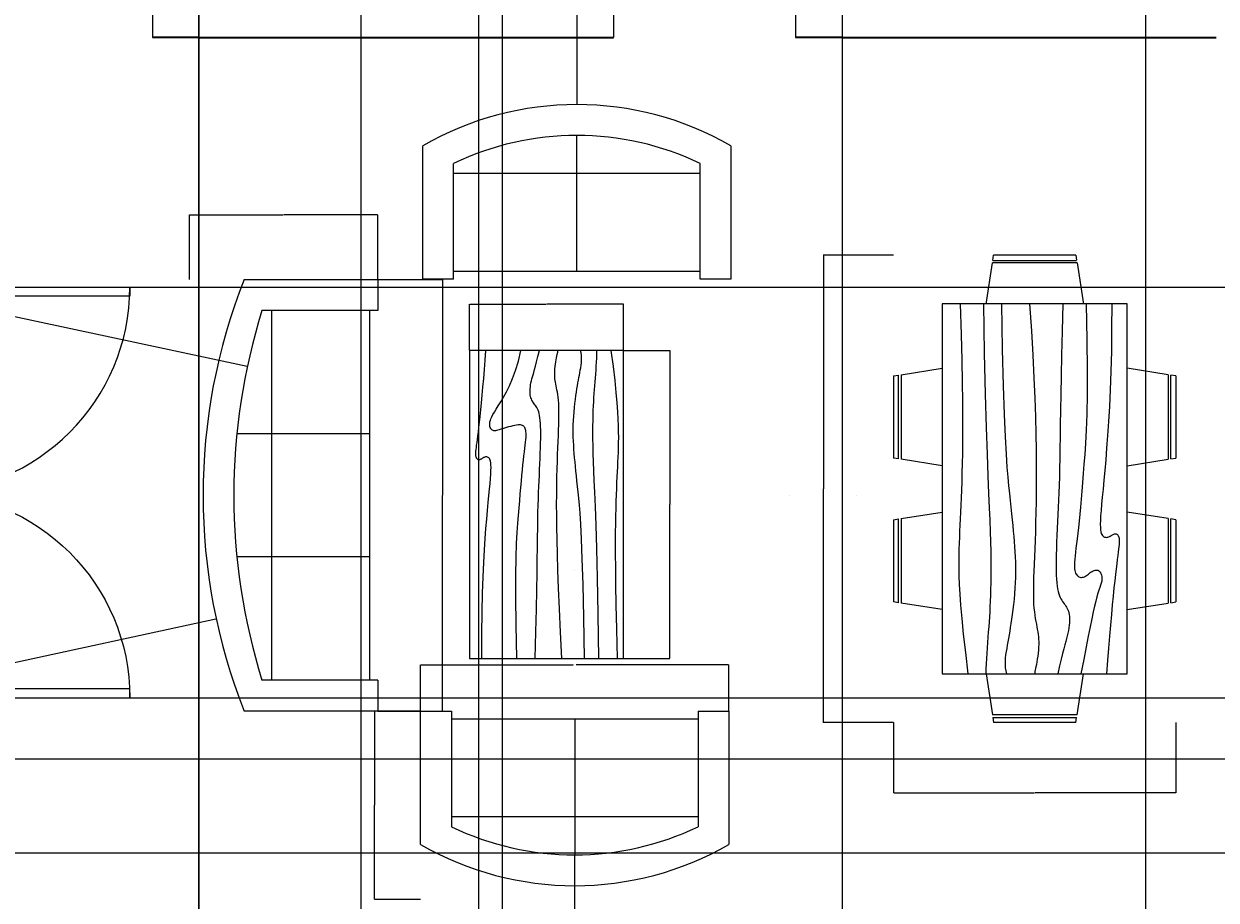
# Model space of a CAD drawing. Units: millimetres. Extents: x -8052 to 19968, y -37825 to -17505.
# Tile 4 of 10: x 84 to 5980, y -29741 to -25407. Entities that reach past the tile are written whole.
import ezdxf

# ---------------------------------------------------------------- set-up
doc = ezdxf.new("R2010")
doc.units = ezdxf.units.MM
doc.header["$MEASUREMENT"] = 0
for name, color, linetype, lineweight in [('A-ANNO-DIMS', 2, 'Continuous', 18), ('A-DOOR', 3, 'Continuous', 25), ('A-FURN', 8, 'Continuous', 18), ('A-WALL', 7, 'Continuous', 35)]:
    doc.layers.add(name, color=color, linetype=linetype, lineweight=lineweight)
doc.styles.get("Standard").update_dxf_attribs({"font": 'arial.ttf'})
doc.dimstyles.get("Standard").update_dxf_attribs({"dimtxt": 1.054, "dimasz": 1.055, "dimexe": 0.18, "dimexo": 0.0625, "dimgap": 0.09, "dimtad": 0, "dimtih": 1, "dimtoh": 1, "dimdec": 4, "dimzin": 0, "dimdsep": 46, "dimtxsty": 'Standard', "dimcen": 0.09, "dimadec": 0, "dimazin": 0, "dimtfac": 1, "dimtdec": 4, "dimtofl": 0, "dimtmove": 0, "dimatfit": 3, "dimfxl": 1, "dimtolj": 1, "dimtzin": 0, "dimarcsym": 0})

# ---------------------------------------------------------------- blocks, each defined once
blk = doc.blocks.new('Dining Set - 36 x 72 in.')
for p, q in [((-22.2343, 26.00059), (-23.4847, 17.99762)), ((-22.2304, 26), (-5.7608, 26)), ((-22, 27.5), (-22.1562, 26.50042)), ((-5.8416, 26.5), (-22.1534, 26.5)), ((-22, 27.5), (-6, 27.5)), ((-5.8437, 26.49966), (-6, 27.5)), ((-4.5152, 17.99762), (-5.7655, 25.99926)), ((5.7657, 26.00059), (4.5153, 17.99762)), ((5.7696, 26), (22.2392, 26)), ((6, 27.5), (5.8438, 26.50042)), ((22.1584, 26.5), (5.8466, 26.5)), ((6, 27.5), (22, 27.5)), ((22.1563, 26.49966), (22, 27.5)), ((23.4848, 17.99762), (22.2345, 25.99926)), ((36, 18), (-36, 18)), ((-36, 18), (-36, -18)), ((36, -18), (36, 18)), ((-44.0006, 8.23428), (-35.9976, 9.48474)), ((44.0006, 8.23428), (35.9976, 9.48474)), ((-45.5, 8), (-44.5004, 8.15617)), ((-45.5, 8), (-45.5, -8)), ((-44.5, -8.15843), (-44.5, 8.15338)), ((-44, 8.23041), (-44, -8.23915)), ((44, 8.23041), (44, -8.23915)), ((44.5, -8.15843), (44.5, 8.15338)), ((45.5, 8), (44.5005, 8.15617)), ((45.5, 8), (45.5, -8)), ((-44.4997, -8.15631), (-45.5, -8)), ((-35.9976, -9.48476), (-43.9993, -8.2345)), ((35.9976, -9.48476), (43.9993, -8.2345)), ((44.4997, -8.15631), (45.5, -8)), ((-36, -18), (36, -18)), ((-22.2343, -26.0006), (-23.4847, -17.99762)), ((-4.5152, -17.99762), (-5.7655, -25.99928)), ((5.7657, -26.0006), (4.5153, -17.99762)), ((23.4848, -17.99762), (22.2345, -25.99928)), ((-22.2304, -26), (-5.7608, -26)), ((-22, -27.5), (-22.1562, -26.50044)), ((-5.8416, -26.5), (-22.1534, -26.5)), ((-22, -27.5), (-6, -27.5)), ((-5.8437, -26.49967), (-6, -27.5)), ((5.7696, -26), (22.2392, -26)), ((6, -27.5), (5.8438, -26.50044)), ((22.1584, -26.5), (5.8466, -26.5)), ((6, -27.5), (22, -27.5)), ((22.1563, -26.49967), (22, -27.5))]:
    blk.add_line(p, q)
for points in [[(-36, 15), (-31.1772, 14.97754), (-26.8079, 14.91406), (-22.8538, 14.81543), (-19.276, 14.6875), (-16.0362, 14.53613), (-13.0957, 14.36718), (-10.4159, 14.18652), (-7.9583, 14), (-5.6904, 13.81315), (-3.6035, 13.63021), (-1.6954, 13.45508), (0.0365, 13.29166), (1.5945, 13.14388), (2.9811, 13.01562), (4.1988, 12.9108), (5.25, 12.83333), (6.1393, 12.78613), (6.8802, 12.76823), (7.4883, 12.77767), (7.9792, 12.8125), (8.3685, 12.87077), (8.6719, 12.95052), (8.9049, 13.0498), (9.0833, 13.16666), (9.2205, 13.29899), (9.3216, 13.44401), (9.3895, 13.59879), (9.4271, 13.76041), (9.4373, 13.92594), (9.4232, 14.09245), (9.3875, 14.257), (9.3333, 14.41666), (9.2638, 14.56917), (9.1836, 14.71484), (9.0975, 14.85465), (9.0104, 14.98958), (8.9272, 15.1206), (8.8529, 15.2487), (8.7922, 15.37483), (8.75, 15.5), (8.7305, 15.62467), (8.7344, 15.74739), (8.7617, 15.86621), (8.8125, 15.97916), (8.8867, 16.08431), (8.9844, 16.17968), (9.1055, 16.26334), (9.25, 16.33333), (9.4189, 16.38802), (9.6172, 16.42708), (9.8506, 16.45052), (10.125, 16.45833), (10.4463, 16.45052), (10.8203, 16.42708), (11.2529, 16.38802), (11.75, 16.33333), (12.3184, 16.26318), (12.9694, 16.17838), (13.7151, 16.07991), (14.5677, 15.96875), (15.5395, 15.84586), (16.6426, 15.71224), (17.8893, 15.56884), (19.2917, 15.41666), (20.859, 15.25667), (22.5879, 15.08984), (24.4721, 14.91715), (26.5052, 14.73958), (28.6809, 14.5581), (30.9929, 14.3737), (33.4347, 14.18733), (36, 14)], [(-36, 10), (-28.9766, 10.14274), (-23.1725, 10.20442), (-18.4241, 10.19775), (-14.5677, 10.13541), (-11.4399, 10.03011), (-8.877, 9.89453), (-6.7154, 9.74137), (-4.7917, 9.58333), (-2.9698, 9.43082), (-1.2246, 9.28515), (0.4415, 9.14534), (2.026, 9.01041), (3.5266, 8.87939), (4.9408, 8.7513), (6.266, 8.62516), (7.5, 8.5), (8.6411, 8.37549), (9.6914, 8.2539), (10.6538, 8.13818), (11.5312, 8.03125), (12.3267, 7.93603), (13.043, 7.85547), (13.6831, 7.79248), (14.25, 7.75), (14.7471, 7.7303), (15.1797, 7.73307), (15.5537, 7.75732), (15.875, 7.80208), (16.1494, 7.86637), (16.3828, 7.94922), (16.5811, 8.04964), (16.75, 8.16666), (16.8944, 8.29915), (17.0143, 8.44531), (17.1089, 8.60319), (17.1771, 8.77083), (17.218, 8.94629), (17.2305, 9.1276), (17.2137, 9.31282), (17.1667, 9.5), (17.0895, 9.6875), (16.987, 9.875), (16.8649, 10.0625), (16.7292, 10.25), (16.5856, 10.4375), (16.4401, 10.625), (16.2985, 10.8125), (16.1667, 11), (16.05, 11.18733), (15.9518, 11.3737), (15.8752, 11.5581), (15.8229, 11.73958), (15.798, 11.91715), (15.8034, 12.08984), (15.842, 12.25667), (15.9167, 12.41666), (16.0295, 12.56836), (16.1784, 12.70833), (16.3605, 12.83268), (16.5729, 12.9375), (16.8127, 13.01888), (17.0768, 13.07291), (17.3625, 13.0957), (17.6667, 13.08333), (17.9894, 13.03312), (18.3418, 12.94726), (18.7382, 12.82918), (19.1927, 12.68229), (19.7195, 12.51001), (20.3327, 12.31575), (21.0465, 12.10294), (21.875, 11.875), (22.8357, 11.63354), (23.959, 11.37304), (25.2786, 11.08618), (26.8282, 10.76562), (28.6414, 10.40405), (30.752, 9.99414), (33.1936, 9.52856), (36, 9)], [(-36, 5.5), (-30.7157, 5.3348), (-26.069, 5.20963), (-21.9946, 5.11767), (-18.4271, 5.05208), (-15.3009, 5.00602), (-12.5508, 4.97265), (-10.1112, 4.94515), (-7.9167, 4.91666), (-5.909, 4.88167), (-4.0586, 4.83984), (-2.3429, 4.79215), (-0.7396, 4.73958), (0.7739, 4.6831), (2.22, 4.6237), (3.6213, 4.56233), (5, 4.5), (6.373, 4.43782), (7.7344, 4.3776), (9.0723, 4.32129), (10.375, 4.27083), (11.6309, 4.22819), (12.8281, 4.19531), (13.9551, 4.17415), (15, 4.16666), (15.954, 4.17448), (16.819, 4.19791), (17.6001, 4.23698), (18.3021, 4.29166), (18.9299, 4.36198), (19.4883, 4.44791), (19.9823, 4.54948), (20.4167, 4.66666), (20.7969, 4.79899), (21.1302, 4.94401), (21.4245, 5.09879), (21.6875, 5.26041), (21.9271, 5.42594), (22.1511, 5.59245), (22.3672, 5.757), (22.5834, 5.91666), (22.8065, 6.06868), (23.0404, 6.21093), (23.2879, 6.34147), (23.5521, 6.45833), (23.8358, 6.55957), (24.142, 6.64323), (24.4735, 6.70735), (24.8334, 6.75), (25.2235, 6.76969), (25.642, 6.76692), (26.0858, 6.74267), (26.5521, 6.69791), (27.0379, 6.63362), (27.5404, 6.55078), (28.0565, 6.45036), (28.5834, 6.33333), (29.1242, 6.19987), (29.7071, 6.04687), (30.3661, 5.87044), (31.1354, 5.66666), (32.0493, 5.43164), (33.142, 5.16146), (34.4475, 4.85221), (36, 4.5)], [(-36, -1), (-30.7915, -0.6591), (-26.0195, -0.38216), (-21.6519, -0.16284), (-17.6563, 0.00521), (-14.0005, 0.12833), (-10.6523, 0.21289), (-7.5796, 0.26522), (-4.75, 0.29166), (-2.134, 0.29793), (0.2878, 0.28711), (2.5317, 0.26163), (4.6146, 0.22396), (6.5529, 0.17651), (8.3633, 0.12174), (10.0623, 0.06209), (11.6667, 0), (13.1899, -0.06201), (14.6341, -0.1211), (15.9982, -0.17432), (17.2813, -0.21875), (18.4823, -0.25147), (19.6003, -0.26953), (20.6343, -0.27002), (21.5834, -0.25), (22.4481, -0.20768), (23.2357, -0.14584), (23.9549, -0.06836), (24.6146, 0.02083), (25.2235, 0.11784), (25.7904, 0.21875), (26.3241, 0.31966), (26.8334, 0.41666), (27.3265, 0.50618), (27.8099, 0.58593), (28.2894, 0.65397), (28.7709, 0.70833), (29.2601, 0.74707), (29.763, 0.76823), (30.2855, 0.76985), (30.8334, 0.75), (31.4088, 0.70784), (31.9994, 0.64713), (32.589, 0.57275), (33.1615, 0.48958), (33.7008, 0.4025), (34.1908, 0.3164), (34.6153, 0.23616), (34.9584, 0.16666), (35.2099, 0.11165), (35.3848, 0.07031), (35.504, 0.04069), (35.5886, 0.02083), (35.6594, 0.00879), (35.7377, 0.0026), (35.8442, 0.00032), (36, 0)], [(-36, -6.5), (-27.1843, -6.31267), (-20.084, -6.1263), (-14.469, -5.9419), (-10.1094, -5.76042), (-6.7752, -5.58285), (-4.2363, -5.41016), (-2.2629, -5.24333), (-0.625, -5.08334), (0.8708, -4.93099), (2.2715, -4.78646), (3.5872, -4.64974), (4.8281, -4.52084), (6.0046, -4.39974), (7.127, -4.28646), (8.2053, -4.18099), (9.25, -4.08334), (10.2705, -3.99382), (11.2734, -3.91407), (12.2647, -3.84603), (13.25, -3.79167), (14.2354, -3.75293), (15.2266, -3.73177), (16.2295, -3.73015), (17.25, -3.75), (18.2912, -3.79248), (19.3451, -3.85547), (20.4009, -3.93604), (21.4479, -4.03125), (22.4754, -4.13819), (23.4727, -4.25391), (24.4289, -4.37549), (25.3334, -4.5), (26.1785, -4.62492), (26.9694, -4.74935), (27.7145, -4.87281), (28.4219, -4.99479), (29.1, -5.11483), (29.7572, -5.23242), (30.4016, -5.34709), (31.0417, -5.45834), (31.6837, -5.56437), (32.3262, -5.65821), (32.9658, -5.73153), (33.599, -5.77604), (34.2224, -5.78345), (34.8327, -5.74545), (35.4264, -5.65373), (36, -5.5)], [(-36, -10), (-26.4022, -9.81299), (-18.4675, -9.62891), (-11.9839, -9.45069), (-6.7396, -9.28125), (-2.5226, -9.12354), (0.8789, -8.98047), (3.6769, -8.85498), (6.0833, -8.75), (8.2767, -8.66765), (10.3021, -8.60677), (12.1712, -8.56543), (13.8958, -8.54167), (15.4876, -8.53353), (16.9583, -8.53907), (18.3197, -8.55632), (19.5834, -8.58334), (20.7616, -8.61841), (21.8685, -8.66081), (22.9188, -8.71004), (23.9271, -8.76563), (24.9081, -8.82707), (25.8763, -8.89388), (26.8465, -8.96558), (27.8334, -9.04167), (28.8474, -9.12118), (29.8828, -9.20117), (30.93, -9.27824), (31.9792, -9.34896), (33.0205, -9.40991), (34.0443, -9.45768), (35.0407, -9.48885), (36, -9.5)], [(-36, -14.5), (-30.0881, -14.33513), (-25.0332, -14.21224), (-20.7312, -14.12647), (-17.0781, -14.07292), (-13.97, -14.04671), (-11.3027, -14.04297), (-8.9724, -14.05681), (-6.875, -14.08334), (-4.9224, -14.11833), (-3.0905, -14.16016), (-1.3709, -14.20785), (0.2448, -14.26042), (1.7647, -14.3169), (3.1973, -14.3763), (4.5507, -14.43767), (5.8333, -14.5), (7.0554, -14.5621), (8.235, -14.62175), (9.3922, -14.67652), (10.5469, -14.72396), (11.7192, -14.76164), (12.929, -14.78711), (14.1965, -14.79794), (15.5417, -14.79167), (16.9933, -14.76424), (18.6152, -14.70508), (20.4804, -14.60197), (22.6615, -14.44271), (25.2312, -14.21509), (28.2624, -13.9069), (31.8277, -13.50594), (36, -13)]]:
    blk.add_lwpolyline(points)
blk = doc.blocks.new('Table - Rectangular Woodgrain 60 x 30 in.')
for p, q in [((0, 0), (0, -30)), ((60, 0), (0, 0)), ((60, -30), (60, 0)), ((0, -30), (60, -30))]:
    blk.add_line(p, q)
for points in [[(0, -2.4), (4.8155, -2.418), (9.0302, -2.4688), (12.709, -2.5477), (15.9167, -2.65), (18.7181, -2.7711), (21.1781, -2.9063), (23.3616, -3.0508), (25.3333, -3.2), (27.1477, -3.3495), (28.8172, -3.4958), (30.3437, -3.636), (31.7291, -3.7667), (32.9756, -3.8849), (34.0849, -3.9875), (35.059, -4.0714), (35.9, -4.1334), (36.6114, -4.1711), (37.2041, -4.1854), (37.6906, -4.1779), (38.0833, -4.15), (38.3948, -4.1034), (38.6375, -4.0396), (38.8239, -3.9602), (38.9666, -3.8667), (39.0764, -3.7608), (39.1573, -3.6448), (39.2116, -3.521), (39.2416, -3.3917), (39.2498, -3.2593), (39.2385, -3.1261), (39.21, -2.9944), (39.1666, -2.8667), (39.111, -2.7447), (39.0468, -2.6281), (38.978, -2.5163), (38.9083, -2.4083), (38.8418, -2.3035), (38.7823, -2.201), (38.7337, -2.1001), (38.7, -2), (38.6844, -1.9003), (38.6875, -1.8021), (38.7094, -1.707), (38.75, -1.6167), (38.8094, -1.5326), (38.8875, -1.4563), (38.9844, -1.3893), (39.1, -1.3333), (39.2351, -1.2896), (39.3937, -1.2583), (39.5804, -1.2396), (39.8, -1.2333), (40.057, -1.2396), (40.3562, -1.2583), (40.7023, -1.2896), (41.1, -1.3333), (41.5547, -1.3895), (42.0755, -1.4573), (42.6721, -1.5361), (43.3542, -1.625), (44.1316, -1.7233), (45.014, -1.8302), (46.0114, -1.9449), (47.1333, -2.0667), (48.3862, -2.1947), (49.7625, -2.3281), (51.2513, -2.4663), (52.8416, -2.6083), (54.5226, -2.7535), (56.2833, -2.9011), (58.1127, -3.0501), (60, -3.2)], [(0, -9.2), (6.5759, -9.0858), (11.9385, -9.0365), (16.2527, -9.0418), (19.6833, -9.0917), (22.3952, -9.1759), (24.5531, -9.2844), (26.322, -9.4069), (27.8666, -9.5333), (29.3241, -9.6553), (30.7203, -9.7719), (32.0532, -9.8837), (33.3208, -9.9917), (34.5213, -10.0965), (35.6526, -10.199), (36.7128, -10.2999), (37.7, -10.4), (38.6129, -10.4996), (39.4531, -10.5969), (40.223, -10.6895), (40.925, -10.775), (41.5613, -10.8512), (42.1344, -10.9156), (42.6465, -10.966), (43.1, -11), (43.4976, -11.0158), (43.8437, -11.0136), (44.143, -10.9942), (44.4, -10.9583), (44.6195, -10.9069), (44.8062, -10.8406), (44.9648, -10.7603), (45.1, -10.6667), (45.2155, -10.5598), (45.3114, -10.4365), (45.3871, -10.2929), (45.4416, -10.125), (45.4743, -9.929), (45.4844, -9.7011), (45.4709, -9.4371), (45.4333, -9.1333), (45.3716, -8.7883), (45.2896, -8.4104), (45.1919, -8.0107), (45.0833, -7.6), (44.9685, -7.1893), (44.8521, -6.7896), (44.7388, -6.4117), (44.6333, -6.0667), (44.54, -5.7628), (44.4614, -5.4979), (44.4001, -5.2675), (44.3583, -5.0667), (44.3384, -4.8909), (44.3427, -4.7354), (44.3736, -4.5956), (44.4333, -4.4667), (44.5236, -4.3453), (44.6427, -4.2333), (44.7884, -4.1339), (44.9583, -4.05), (45.1501, -3.9849), (45.3614, -3.9417), (45.59, -3.9234), (45.8333, -3.9333), (46.0915, -3.9749), (46.3734, -4.0531), (46.6906, -4.1736), (47.0542, -4.3417), (47.4756, -4.5629), (47.9661, -4.8427), (48.5372, -5.1866), (49.2, -5.6), (49.9676, -6.0844), (50.8594, -6.625), (51.8965, -7.2031), (53.1, -7.8), (54.491, -8.3969), (56.0906, -8.975), (57.9199, -9.5156), (60, -10)], [(0, -12.8), (5.1847, -12.9322), (9.6213, -13.0323), (13.3963, -13.1059), (16.5958, -13.1583), (19.3063, -13.1952), (21.614, -13.2219), (23.6054, -13.2439), (25.3666, -13.2667), (26.9728, -13.2947), (28.4531, -13.3281), (29.8256, -13.3663), (31.1083, -13.4083), (32.3191, -13.4535), (33.476, -13.501), (34.597, -13.5501), (35.7, -13.6), (36.7984, -13.6497), (37.8875, -13.6979), (38.9578, -13.743), (40, -13.7833), (41.0047, -13.8174), (41.9625, -13.8438), (42.864, -13.8607), (43.7, -13.8667), (44.4631, -13.8604), (45.1552, -13.8417), (45.7801, -13.8104), (46.3416, -13.7667), (46.8439, -13.7104), (47.2906, -13.6417), (47.6858, -13.5604), (48.0333, -13.4667), (48.3375, -13.3608), (48.6042, -13.2448), (48.8396, -13.121), (49.05, -12.9917), (49.2417, -12.8593), (49.4208, -12.7261), (49.5937, -12.5944), (49.7667, -12.4667), (49.9452, -12.3451), (50.1323, -12.2313), (50.3303, -12.1268), (50.5416, -12.0333), (50.7686, -11.9524), (51.0135, -11.8854), (51.2788, -11.8341), (51.5666, -11.8), (51.8785, -11.7843), (52.2116, -11.7865), (52.562, -11.8059), (52.926, -11.8417), (53.2998, -11.8931), (53.6795, -11.9594), (54.0614, -12.0397), (54.4416, -12.1333), (54.8223, -12.2401), (55.2293, -12.3625), (55.6942, -12.5037), (56.2489, -12.6667), (56.9251, -12.8547), (57.7545, -13.0708), (58.7689, -13.3182), (60, -13.6)], [(0, -18), (5.124, -17.7273), (9.6609, -17.5057), (13.6705, -17.3303), (17.2125, -17.1958), (20.3467, -17.0973), (23.1328, -17.0297), (25.6307, -16.9878), (27.9, -16.9667), (29.9928, -16.9617), (31.9302, -16.9703), (33.7254, -16.9907), (35.3917, -17.0208), (36.9423, -17.0588), (38.3906, -17.1026), (39.7499, -17.1503), (41.0333, -17.2), (42.2519, -17.2496), (43.4073, -17.2969), (44.4986, -17.3395), (45.525, -17.375), (46.4858, -17.4012), (47.3802, -17.4156), (48.2074, -17.416), (48.9667, -17.4), (49.6583, -17.3662), (50.2872, -17.3167), (50.8595, -17.2547), (51.3812, -17.1833), (51.8584, -17.1057), (52.2971, -17.025), (52.7034, -16.9443), (53.0833, -16.8667), (53.443, -16.7951), (53.789, -16.7313), (54.128, -16.6768), (54.4666, -16.6334), (54.8115, -16.6024), (55.1693, -16.5854), (55.5465, -16.5841), (55.95, -16.6), (56.3828, -16.6337), (56.8346, -16.6823), (57.2915, -16.7418), (57.7396, -16.8084), (58.165, -16.878), (58.5539, -16.9469), (58.8924, -17.0111), (59.1666, -17.0667), (59.3679, -17.1107), (59.5078, -17.1438), (59.6032, -17.1675), (59.6708, -17.1833), (59.7275, -17.193), (59.7901, -17.1979), (59.8753, -17.1998), (60, -17.2)], [(0, -22.4), (8.0098, -22.2501), (14.4094, -22.1011), (19.4168, -21.9535), (23.25, -21.8083), (26.1269, -21.6663), (28.2656, -21.5281), (29.884, -21.3947), (31.2, -21.2667), (32.3967, -21.1448), (33.5172, -21.0292), (34.5697, -20.9198), (35.5625, -20.8167), (36.5037, -20.7198), (37.4015, -20.6292), (38.2642, -20.5448), (39.1, -20.4667), (39.9164, -20.3951), (40.7187, -20.3313), (41.5117, -20.2768), (42.3, -20.2333), (43.0883, -20.2024), (43.8812, -20.1854), (44.6836, -20.1841), (45.5, -20.2), (46.3328, -20.234), (47.1747, -20.2844), (48.0163, -20.3488), (48.8479, -20.425), (49.66, -20.5106), (50.4429, -20.6031), (51.1872, -20.7004), (51.8833, -20.8), (52.5246, -20.8999), (53.1166, -20.9995), (53.6681, -21.0983), (54.1875, -21.1958), (54.6834, -21.2919), (55.1646, -21.3859), (55.6394, -21.4777), (56.1167, -21.5667), (56.6028, -21.6515), (57.0961, -21.7266), (57.5929, -21.7852), (58.0896, -21.8208), (58.5823, -21.8268), (59.0674, -21.7964), (59.5412, -21.723), (60, -21.6)], [(0, -25.2), (8.6355, -25.0504), (15.7026, -24.9031), (21.4049, -24.7606), (25.9458, -24.625), (29.529, -24.4988), (32.3578, -24.3844), (34.6359, -24.284), (36.5667, -24.2), (38.3213, -24.1341), (39.9417, -24.0854), (41.437, -24.0523), (42.8167, -24.0333), (44.0901, -24.0268), (45.2667, -24.0313), (46.3557, -24.0451), (47.3667, -24.0667), (48.309, -24.0947), (49.1928, -24.1287), (50.0284, -24.168), (50.826, -24.2125), (51.5959, -24.2617), (52.3483, -24.3151), (53.0935, -24.3725), (53.8417, -24.4334), (54.6009, -24.497), (55.3699, -24.561), (56.1454, -24.6226), (56.9239, -24.6792), (57.7021, -24.7279), (58.4764, -24.7662), (59.2435, -24.7911), (60, -24.8)], [(0, -28.8), (5.6867, -28.6681), (10.45, -28.5698), (14.407, -28.5012), (17.675, -28.4584), (20.3711, -28.4374), (22.6125, -28.4344), (24.5164, -28.4455), (26.2, -28.4667), (27.762, -28.4947), (29.2276, -28.5281), (30.6033, -28.5663), (31.8958, -28.6084), (33.1118, -28.6535), (34.2578, -28.7011), (35.3405, -28.7501), (36.3666, -28.8), (37.3443, -28.8497), (38.288, -28.8974), (39.2137, -28.9412), (40.1375, -28.9792), (41.0753, -29.0093), (42.0432, -29.0297), (43.0572, -29.0384), (44.1333, -29.0333), (45.2936, -29.0114), (46.5843, -28.9641), (48.0579, -28.8816), (49.7666, -28.7542), (51.7629, -28.5721), (54.0989, -28.3255), (56.8272, -28.0048), (60, -27.6)]]:
    blk.add_lwpolyline(points)
blk = doc.blocks.new('Sofa - Roundback Loveseat 5 ft.')
for p, q in [((0, -32.44198), (0, -5.99998)), ((-24, -33.99998), (-24, -11.46958)), ((24.00004, -33.99998), (24.00004, -11.46958)), ((-23.9998, -13.38178), (23.99986, -13.38178)), ((-24, -32.44198), (24.00004, -32.44198))]:
    blk.add_line(p, q)
for points in [[(-24, -33.99998), (-30, -33.99998), (-30, -7.99998)], [(30.00004, -7.99998), (30.00004, -33.99998), (24.00004, -33.99998)]]:
    blk.add_lwpolyline(points)
for centre, radius, start, end in [((0, -60.24998), 60.24998, 60.13715, 119.8628), ((0, -61.38438), 55.38444, 64.32083, 115.6792)]:
    blk.add_arc(centre, radius, start, end)
blk = doc.blocks.new('Sofa - Roundback 7 ft.')
for p, q in [((-12.00002, -32.4421), (-12.00003, -6.5971)), ((11.99997, -32.4421), (11.99998, -6.5971)), ((-36.000027, -34), (-36.000027, -11.4696)), ((35.99998, -34), (35.99998, -11.4696)), ((-35.999844, -13.3819), (35.9998, -13.3819)), ((-36.000027, -32.4421), (35.99998, -32.4421))]:
    blk.add_line(p, q)
for points in [[(-36.000027, -34), (-42.000027, -34), (-42.000027, -8)], [(41.99998, -8), (41.99998, -34), (35.99998, -34)]]:
    blk.add_lwpolyline(points)
for centre, radius, start, end in [((0, -114.25), 114.25, 68.43141, 111.5686), ((-0.00001, -127.1968), 121.1968, 72.72033, 107.2797)]:
    blk.add_arc(centre, radius, start, end)
blk = doc.blocks.new('*U21')
for p, q in [((0, 0), (0, -6)), ((40, 0), (40, -6))]:
    blk.add_line(p, q)
blk.add_lwpolyline([(0, 0), (0, 40), (1.75, 40), (1.75, 0)], close=True)
blk.add_arc((0, 0), 40, 0, 90)
blk = doc.blocks.new('*D58')
at = {"layer": 'A-ANNO-DIMS', "color": 0, "lineweight": -2, "transparency": 16777216}
for p, q in [((2046.2, -28805.6), (2046.2, -28576.9)), ((2047.3, -28577.1), (2800.7, -28577.1)), ((3569.1, -28577.1), (2815.7, -28577.1)), ((3570.2, -28805.6), (3570.2, -28576.9))]:
    blk.add_line(p, q, dxfattribs=at)
at = {"layer": 'A-ANNO-DIMS', "color": 0, "lineweight": 100, "transparency": 16777216}
for points in [[(2047.3, -28576.9), (2047.3, -28577.3), (2046.2, -28577.1)], [(3569.1, -28576.9), (3569.1, -28577.3), (3570.2, -28577.1)]]:
    blk.add_solid(points, dxfattribs=at)
at = {"layer": 'Defpoints', "color": 0, "lineweight": 100, "transparency": 16777216}
for p in [(2046.2, -28577.1), (2046.2, -28805.7), (3570.2, -28805.7)]:
    blk.add_point(p, dxfattribs=at)
at = {"layer": 'A-ANNO-DIMS', "color": 0, "transparency": 16777216, "insert": (2808.2, -28577.1), "char_height": 1.054, "attachment_point": 5}
blk.add_mtext('\\A1;LOVESEAT 1524 TYP.', dxfattribs=at)
blk = doc.blocks.new('*D59')
at = {"layer": 'A-ANNO-DIMS', "color": 0, "lineweight": -2, "transparency": 16777216}
for p, q in [((2046.1, -28805.7), (1817.4, -28805.7)), ((1817.6, -28806.7), (1817.6, -29270.7)), ((1817.6, -29736), (1817.6, -29272)), ((2046.1, -29737), (1817.4, -29737))]:
    blk.add_line(p, q, dxfattribs=at)
at = {"layer": 'A-ANNO-DIMS', "color": 0, "lineweight": 100, "transparency": 16777216}
for points in [[(1817.4, -28806.7), (1817.8, -28806.7), (1817.6, -28805.7)], [(1817.4, -29736), (1817.8, -29736), (1817.6, -29737)]]:
    blk.add_solid(points, dxfattribs=at)
at = {"layer": 'Defpoints', "color": 0, "lineweight": 100, "transparency": 16777216}
for p in [(2046.2, -28805.7), (1817.6, -29737), (2046.2, -29737)]:
    blk.add_point(p, dxfattribs=at)
at = {"layer": 'A-ANNO-DIMS', "color": 0, "transparency": 16777216, "insert": (1817.6, -29271.4), "char_height": 1.054, "attachment_point": 5}
blk.add_mtext('\\A1;931 TYP.', dxfattribs=at)
blk = doc.blocks.new('*D70')
at = {"layer": 'A-ANNO-DIMS', "color": 0, "lineweight": -2, "transparency": 16777216}
for p, q in [((4384.3, -26551.5), (4037.5, -26551.5)), ((4037.6, -26552.5), (4037.6, -27706.5)), ((4037.6, -28861.8), (4037.6, -27707.8)), ((4384.3, -28862.9), (4037.5, -28862.9))]:
    blk.add_line(p, q, dxfattribs=at)
at = {"layer": 'A-ANNO-DIMS', "color": 0, "lineweight": 100, "transparency": 16777216}
for points in [[(4037.5, -26552.5), (4037.8, -26552.5), (4037.6, -26551.5)], [(4037.5, -28861.8), (4037.8, -28861.8), (4037.6, -28862.9)]]:
    blk.add_solid(points, dxfattribs=at)
at = {"layer": 'Defpoints', "color": 0, "lineweight": 100, "transparency": 16777216}
for p in [(4384.3, -26551.5), (4037.6, -28862.9), (4384.3, -28862.9)]:
    blk.add_point(p, dxfattribs=at)
at = {"layer": 'A-ANNO-DIMS', "color": 0, "transparency": 16777216, "insert": (4037.6, -27707.2), "char_height": 1.054, "attachment_point": 5}
blk.add_mtext('\\A1;DINING SET 2311', dxfattribs=at)
blk = doc.blocks.new('*D71')
at = {"layer": 'A-ANNO-DIMS', "color": 0, "lineweight": -2, "transparency": 16777216}
for p, q in [((4384.3, -28862.9), (4384.3, -29209.8)), ((5781.3, -28862.9), (5781.3, -29209.8)), ((4385.4, -29209.6), (5081.2, -29209.6)), ((5780.3, -29209.6), (5084.5, -29209.6))]:
    blk.add_line(p, q, dxfattribs=at)
at = {"layer": 'A-ANNO-DIMS', "color": 0, "lineweight": 100, "transparency": 16777216}
for points in [[(4385.4, -29209.4), (4385.4, -29209.8), (4384.3, -29209.6)], [(5780.3, -29209.4), (5780.3, -29209.8), (5781.3, -29209.6)]]:
    blk.add_solid(points, dxfattribs=at)
at = {"layer": 'Defpoints', "color": 0, "lineweight": 100, "transparency": 16777216}
for p in [(4384.3, -28862.9), (5781.3, -28862.9), (5781.3, -29209.6)]:
    blk.add_point(p, dxfattribs=at)
at = {"layer": 'A-ANNO-DIMS', "color": 0, "transparency": 16777216, "insert": (5082.8, -29209.6), "char_height": 1.05, "attachment_point": 5}
blk.add_mtext('\\A1;1397', dxfattribs=at)
blk = doc.blocks.new('*D72')
at = {"layer": 'A-ANNO-DIMS', "color": 0, "lineweight": -2, "transparency": 16777216}
for p, q in [((3050, -27022), (3278.8, -27022)), ((3278.6, -27023), (3278.6, -27783.3)), ((3278.6, -28544.9), (3278.6, -27784.6)), ((3050, -28546), (3278.8, -28546))]:
    blk.add_line(p, q, dxfattribs=at)
at = {"layer": 'A-ANNO-DIMS', "color": 0, "lineweight": 100, "transparency": 16777216}
for points in [[(3278.4, -27023), (3278.8, -27023), (3278.6, -27022)], [(3278.4, -28544.9), (3278.8, -28544.9), (3278.6, -28546)]]:
    blk.add_solid(points, dxfattribs=at)
at = {"layer": 'Defpoints', "color": 0, "lineweight": 100, "transparency": 16777216}
for p in [(3050, -27022), (3278.6, -27022), (3050, -28546)]:
    blk.add_point(p, dxfattribs=at)
at = {"layer": 'A-ANNO-DIMS', "color": 0, "transparency": 16777216, "insert": (3278.6, -27784), "char_height": 1.054, "attachment_point": 5}
blk.add_mtext('\\A1;COFFEE TABLE 1524', dxfattribs=at)
blk = doc.blocks.new('*D73')
at = {"layer": 'A-ANNO-DIMS', "color": 0, "lineweight": -2, "transparency": 16777216}
for p, q in [((2288, -27021.9), (2288, -26793.2)), ((2289, -26793.4), (2667.7, -26793.4)), ((3048.9, -26793.4), (2670.2, -26793.4)), ((3050, -27021.9), (3050, -26793.2))]:
    blk.add_line(p, q, dxfattribs=at)
at = {"layer": 'A-ANNO-DIMS', "color": 0, "lineweight": 100, "transparency": 16777216}
for points in [[(2289, -26793.2), (2289, -26793.5), (2288, -26793.4)], [(3048.9, -26793.2), (3048.9, -26793.5), (3050, -26793.4)]]:
    blk.add_solid(points, dxfattribs=at)
at = {"layer": 'Defpoints', "color": 0, "lineweight": 100, "transparency": 16777216}
for p in [(2288, -26793.4), (2288, -27022), (3050, -27022)]:
    blk.add_point(p, dxfattribs=at)
at = {"layer": 'A-ANNO-DIMS', "color": 0, "transparency": 16777216, "insert": (2669, -26793.4), "char_height": 1.05, "attachment_point": 5}
blk.add_mtext('\\A1;762', dxfattribs=at)
blk = doc.blocks.new('*D74')
at = {"layer": 'A-ANNO-DIMS', "color": 0, "lineweight": -2, "transparency": 16777216}
for p, q in [((1834, -26672.1), (2154.1, -26672.1)), ((2154, -26673.1), (2154, -27738.3)), ((2154, -28804.6), (2154, -27739.5)), ((1834, -28805.7), (2154.1, -28805.7))]:
    blk.add_line(p, q, dxfattribs=at)
at = {"layer": 'A-ANNO-DIMS', "color": 0, "lineweight": 100, "transparency": 16777216}
for points in [[(2153.8, -26673.1), (2154.1, -26673.1), (2154, -26672.1)], [(2153.8, -28804.6), (2154.1, -28804.6), (2154, -28805.7)]]:
    blk.add_solid(points, dxfattribs=at)
at = {"layer": 'Defpoints', "color": 0, "lineweight": 100, "transparency": 16777216}
for p in [(1833.9, -26672.1), (2154, -26672.1), (1833.9, -28805.7)]:
    blk.add_point(p, dxfattribs=at)
at = {"layer": 'A-ANNO-DIMS', "color": 0, "transparency": 16777216, "insert": (2154, -27738.9), "char_height": 1.054, "attachment_point": 5}
blk.add_mtext('\\A1;SOFA 2134', dxfattribs=at)
blk = doc.blocks.new('*D75')
at = {"layer": 'A-ANNO-DIMS', "color": 0, "lineweight": -2, "transparency": 16777216}
for p, q in [((902.6, -26672), (902.6, -26351.9)), ((903.6, -26352), (1367.1, -26352)), ((1832.9, -26352), (1369.4, -26352)), ((1833.9, -26672), (1833.9, -26351.9))]:
    blk.add_line(p, q, dxfattribs=at)
at = {"layer": 'A-ANNO-DIMS', "color": 0, "lineweight": 100, "transparency": 16777216}
for points in [[(903.6, -26351.9), (903.6, -26352.2), (902.6, -26352)], [(1832.9, -26351.9), (1832.9, -26352.2), (1833.9, -26352)]]:
    blk.add_solid(points, dxfattribs=at)
at = {"layer": 'Defpoints', "color": 0, "lineweight": 100, "transparency": 16777216}
for p in [(902.6, -26352), (902.6, -26672.1), (1833.9, -26672.1)]:
    blk.add_point(p, dxfattribs=at)
at = {"layer": 'A-ANNO-DIMS', "color": 0, "transparency": 16777216, "insert": (1368.3, -26352), "char_height": 1.05, "attachment_point": 5}
blk.add_mtext('\\A1;931', dxfattribs=at)
blk = doc.blocks.new('*D95')
at = {"layer": 'A-ANNO-DIMS', "color": 0, "lineweight": -2, "transparency": 16777216}
for p, q in [((4130, -20744.9), (4130, -37824.5)), ((5630, -20744.9), (5630, -37824.5)), ((4131, -37824.3), (4878.4, -37824.3)), ((5628.9, -37824.3), (4881.6, -37824.3))]:
    blk.add_line(p, q, dxfattribs=at)
at = {"layer": 'A-ANNO-DIMS', "color": 0, "lineweight": 100, "transparency": 16777216}
for points in [[(4131, -37824.2), (4131, -37824.5), (4130, -37824.3)], [(5628.9, -37824.2), (5628.9, -37824.5), (5630, -37824.3)]]:
    blk.add_solid(points, dxfattribs=at)
at = {"layer": 'Defpoints', "color": 0, "lineweight": 100, "transparency": 16777216}
for p in [(4130, -20744.8), (5630, -20744.8), (5630, -37824.3)]:
    blk.add_point(p, dxfattribs=at)
at = {"layer": 'A-ANNO-DIMS', "color": 0, "transparency": 16777216, "insert": (4880, -37824.3), "char_height": 1.05, "attachment_point": 5}
blk.add_mtext('\\A1;1500', dxfattribs=at)
blk = doc.blocks.new('*D108')
at = {"layer": 'A-ANNO-DIMS', "color": 0, "lineweight": -2, "transparency": 16777216}
for p, q in [((-330, -29974.8), (-330, -17505.2)), ((-329, -17505.3), (3348.3, -17505.3)), ((7028.9, -17505.3), (3351.6, -17505.3)), ((7030, -29974.8), (7030, -17505.2))]:
    blk.add_line(p, q, dxfattribs=at)
at = {"layer": 'A-ANNO-DIMS', "color": 0, "lineweight": 100, "transparency": 16777216}
for points in [[(-329, -17505.2), (-329, -17505.5), (-330, -17505.3)], [(7028.9, -17505.2), (7028.9, -17505.5), (7030, -17505.3)]]:
    blk.add_solid(points, dxfattribs=at)
at = {"layer": 'Defpoints', "color": 0, "lineweight": 100, "transparency": 16777216}
for p in [(7030, -17505.3), (-330, -29974.8), (7030, -29974.8)]:
    blk.add_point(p, dxfattribs=at)
at = {"layer": 'A-ANNO-DIMS', "color": 0, "transparency": 16777216, "insert": (3350, -17505.3), "char_height": 1.05, "attachment_point": 5}
blk.add_mtext('\\A1;7360', dxfattribs=at)
blk = doc.blocks.new('*D111')
at = {"layer": 'A-ANNO-DIMS', "color": 0, "lineweight": -2, "transparency": 16777216}
for p, q in [((-560, -26708.8), (14099.7, -26708.8)), ((14099.5, -26709.9), (14099.5, -27724.2)), ((14099.5, -28739.8), (14099.5, -27725.5)), ((-560, -28740.8), (14099.7, -28740.8))]:
    blk.add_line(p, q, dxfattribs=at)
at = {"layer": 'A-ANNO-DIMS', "color": 0, "lineweight": 100, "transparency": 16777216}
for points in [[(14099.3, -26709.9), (14099.7, -26709.9), (14099.5, -26708.8)], [(14099.3, -28739.8), (14099.7, -28739.8), (14099.5, -28740.8)]]:
    blk.add_solid(points, dxfattribs=at)
at = {"layer": 'Defpoints', "color": 0, "lineweight": 100, "transparency": 16777216}
for p in [(-560, -26708.8), (-560, -28740.8), (14099.5, -28740.8)]:
    blk.add_point(p, dxfattribs=at)
at = {"layer": 'A-ANNO-DIMS', "color": 0, "transparency": 16777216, "insert": (14099.5, -27724.8), "char_height": 1.05, "attachment_point": 5}
blk.add_mtext('\\A1;2032', dxfattribs=at)
blk = doc.blocks.new('*D112')
at = {"layer": 'A-ANNO-DIMS', "color": 0, "lineweight": -2, "transparency": 16777216}
for p, q in [((8883.8, -29042.9), (-8049.7, -29042.9)), ((-8049.5, -29043.9), (-8049.5, -29275.2)), ((-8049.5, -29507.8), (-8049.5, -29276.5)), ((8883.8, -29508.9), (-8049.7, -29508.9))]:
    blk.add_line(p, q, dxfattribs=at)
at = {"layer": 'A-ANNO-DIMS', "color": 0, "lineweight": 100, "transparency": 16777216}
for points in [[(-8049.7, -29043.9), (-8049.3, -29043.9), (-8049.5, -29042.9)], [(-8049.7, -29507.8), (-8049.3, -29507.8), (-8049.5, -29508.9)]]:
    blk.add_solid(points, dxfattribs=at)
at = {"layer": 'Defpoints', "color": 0, "lineweight": 100, "transparency": 16777216}
for p in [(8883.8, -29042.9), (-8049.5, -29508.9), (8883.8, -29508.9)]:
    blk.add_point(p, dxfattribs=at)
at = {"layer": 'A-ANNO-DIMS', "color": 0, "transparency": 16777216, "insert": (-8049.5, -29275.9), "char_height": 1.05, "attachment_point": 5}
blk.add_mtext('\\A1;466', dxfattribs=at)
blk = doc.blocks.new('*D113')
at = {"layer": 'A-ANNO-DIMS', "color": 0, "lineweight": -2, "transparency": 16777216}
for p, q in [((950, -25244.9), (950, -37824.5)), ((1750, -25244.9), (1750, -37824.5)), ((951, -37824.3), (1348.7, -37824.3)), ((1748.9, -37824.3), (1351.2, -37824.3))]:
    blk.add_line(p, q, dxfattribs=at)
at = {"layer": 'A-ANNO-DIMS', "color": 0, "lineweight": 100, "transparency": 16777216}
for points in [[(951, -37824.2), (951, -37824.5), (950, -37824.3)], [(1748.9, -37824.2), (1748.9, -37824.5), (1750, -37824.3)]]:
    blk.add_solid(points, dxfattribs=at)
at = {"layer": 'Defpoints', "color": 0, "lineweight": 100, "transparency": 16777216}
for p in [(950, -25244.8), (1750, -25244.8), (1750, -37824.3)]:
    blk.add_point(p, dxfattribs=at)
at = {"layer": 'A-ANNO-DIMS', "color": 0, "transparency": 16777216, "insert": (1350, -37824.3), "char_height": 1.05, "attachment_point": 5}
blk.add_mtext('\\A1;800', dxfattribs=at)
blk = doc.blocks.new('*D115')
at = {"layer": 'A-ANNO-DIMS', "color": 0, "lineweight": -2, "transparency": 16777216}
for p, q in [((950, -20744.9), (950, -37824.5)), ((2450, -20744.9), (2450, -37824.5)), ((951, -37824.3), (1698.4, -37824.3)), ((2448.9, -37824.3), (1701.6, -37824.3))]:
    blk.add_line(p, q, dxfattribs=at)
at = {"layer": 'A-ANNO-DIMS', "color": 0, "lineweight": 100, "transparency": 16777216}
for points in [[(951, -37824.2), (951, -37824.5), (950, -37824.3)], [(2448.9, -37824.2), (2448.9, -37824.5), (2450, -37824.3)]]:
    blk.add_solid(points, dxfattribs=at)
at = {"layer": 'Defpoints', "color": 0, "lineweight": 100, "transparency": 16777216}
for p in [(950, -20744.8), (2450, -20744.8), (2450, -37824.3)]:
    blk.add_point(p, dxfattribs=at)
at = {"layer": 'A-ANNO-DIMS', "color": 0, "transparency": 16777216, "insert": (1700, -37824.3), "char_height": 1.05, "attachment_point": 5}
blk.add_mtext('\\A1;1500', dxfattribs=at)
blk = doc.blocks.new('*D118')
at = {"layer": 'A-ANNO-DIMS', "color": 0, "lineweight": -2, "transparency": 16777216}
for p, q in [((950, -33624.8), (950, -17505.2)), ((951, -17505.3), (1640.4, -17505.3)), ((2332.9, -17505.3), (1643.6, -17505.3)), ((2334, -33624.8), (2334, -17505.2))]:
    blk.add_line(p, q, dxfattribs=at)
at = {"layer": 'A-ANNO-DIMS', "color": 0, "lineweight": 100, "transparency": 16777216}
for points in [[(951, -17505.2), (951, -17505.5), (950, -17505.3)], [(2332.9, -17505.2), (2332.9, -17505.5), (2334, -17505.3)]]:
    blk.add_solid(points, dxfattribs=at)
at = {"layer": 'Defpoints', "color": 0, "lineweight": 100, "transparency": 16777216}
for p in [(2334, -17505.3), (950, -33624.8), (2334, -33624.8)]:
    blk.add_point(p, dxfattribs=at)
at = {"layer": 'A-ANNO-DIMS', "color": 0, "transparency": 16777216, "insert": (1642, -17505.3), "char_height": 1.05, "attachment_point": 5}
blk.add_mtext('\\A1;1384', dxfattribs=at)
blk = doc.blocks.new('*D133')
at = {"layer": 'A-ANNO-DIMS', "color": 0, "lineweight": -2, "transparency": 16777216}
for p, q in [((-617, -26716.3), (1188.8, -27099.5)), ((4201, -27738.9), (4201.2, -27738.9)), ((4201.1, -27739), (4201.1, -27738.8))]:
    blk.add_line(p, q, dxfattribs=at)
at = {"layer": 'A-ANNO-DIMS', "color": 0, "lineweight": 100, "transparency": 16777216}
blk.add_solid([(1188.8, -27099.4), (1188.7, -27099.7), (1189.8, -27099.7)], dxfattribs=at)
at = {"layer": 'Defpoints', "color": 0, "lineweight": 100, "transparency": 16777216}
for p in [(1189.8, -27099.7), (4201.1, -27738.9)]:
    blk.add_point(p, dxfattribs=at)
at = {"layer": 'A-ANNO-DIMS', "color": 0, "transparency": 16777216, "insert": (-619.8, -26716.3), "char_height": 1.054, "attachment_point": 5}
blk.add_mtext('\\A1;R3078.4', dxfattribs=at)
blk = doc.blocks.new('*D134')
at = {"layer": 'A-ANNO-DIMS', "color": 0, "lineweight": -2, "transparency": 16777216}
for p, q in [((3872.2, -27738.9), (3872.4, -27738.9)), ((3872.3, -27739), (3872.3, -27738.8)), ((-666.8, -28716.5), (1034.3, -28350.1))]:
    blk.add_line(p, q, dxfattribs=at)
at = {"layer": 'A-ANNO-DIMS', "color": 0, "lineweight": 100, "transparency": 16777216}
blk.add_solid([(1034.3, -28350), (1034.4, -28350.3), (1035.4, -28349.9)], dxfattribs=at)
at = {"layer": 'Defpoints', "color": 0, "lineweight": 100, "transparency": 16777216}
for p in [(3872.3, -27738.9), (1035.4, -28349.9)]:
    blk.add_point(p, dxfattribs=at)
at = {"layer": 'A-ANNO-DIMS', "color": 0, "transparency": 16777216, "insert": (-668.9, -28716.5), "char_height": 1.05, "attachment_point": 5}
blk.add_mtext('\\A1;R2902', dxfattribs=at)
blk = doc.blocks.new('*D135')
at = {"layer": 'A-ANNO-DIMS', "color": 0, "lineweight": -2, "transparency": 16777216}
for p, q in [((2819.8, -24888.5), (2818.7, -24888.5)), ((2818.7, -24888.5), (2818.7, -25805.6)), ((2818.7, -27337), (2818.8, -27337)), ((2818.7, -27337.1), (2818.7, -27337))]:
    blk.add_line(p, q, dxfattribs=at)
at = {"layer": 'A-ANNO-DIMS', "color": 0, "lineweight": 100, "transparency": 16777216}
blk.add_solid([(2818.6, -25805.6), (2818.9, -25805.6), (2818.7, -25806.7)], dxfattribs=at)
at = {"layer": 'Defpoints', "color": 0, "lineweight": 100, "transparency": 16777216}
for p in [(2818.7, -25806.7), (2818.7, -27337)]:
    blk.add_point(p, dxfattribs=at)
at = {"layer": 'A-ANNO-DIMS', "color": 0, "transparency": 16777216, "insert": (2823.7, -24888.5), "char_height": 1.054, "attachment_point": 5}
blk.add_mtext('\\A1;2X R1530.3', dxfattribs=at)
blk = doc.blocks.new('*D136')
at = {"layer": 'A-ANNO-DIMS', "color": 0, "lineweight": -2, "transparency": 16777216}
for p, q in [((2808.1, -28110.1), (2808.3, -28110.1)), ((2808.2, -28110.2), (2808.2, -28110)), ((2808.2, -30360.9), (2808.2, -29517.9)), ((2807.1, -30360.9), (2808.2, -30360.9))]:
    blk.add_line(p, q, dxfattribs=at)
at = {"layer": 'A-ANNO-DIMS', "color": 0, "lineweight": 100, "transparency": 16777216}
blk.add_solid([(2808, -29517.9), (2808.4, -29517.9), (2808.2, -29516.9)], dxfattribs=at)
at = {"layer": 'Defpoints', "color": 0, "lineweight": 100, "transparency": 16777216}
for p in [(2808.2, -28110.1), (2808.2, -29516.9)]:
    blk.add_point(p, dxfattribs=at)
at = {"layer": 'A-ANNO-DIMS', "color": 0, "transparency": 16777216, "insert": (2803.2, -30360.9), "char_height": 1.054, "attachment_point": 5}
blk.add_mtext('\\A1;2X R1406.8', dxfattribs=at)

msp = doc.modelspace()

# ---------------------------------------------------------------- linework, layer by layer
at = {"layer": 'A-DOOR'}
for p, q in [((719.979, -25317.343), (719.979, -25474.843)), ((2999.979, -25339.843), (2999.979, -25474.843)), ((3899.979, -25339.843), (3899.979, -25474.843))]:
    msp.add_line(p, q, dxfattribs=at)
at = {"layer": 'A-WALL'}
for p, q in [((949.979, -25474.843), (719.979, -25474.843)), ((949.979, -25474.843), (2999.979, -25474.843)), ((4129.979, -25474.843), (3899.979, -25474.843)), ((4129.979, -25474.843), (5579.979, -25474.843)), ((5579.979, -25474.843), (5979.979, -25474.843))]:
    msp.add_line(p, q, dxfattribs=at)

# ---------------------------------------------------------------- block references
at = {"layer": 'A-DOOR', "yscale": 25.4, "zscale": 25.4, "rotation": 270}
for p, xscale in [((-407.621, -26708.843), 25.4), ((-407.621, -28740.843), -25.4)]:
    msp.add_blockref('*U21', p, dxfattribs=dict(at, xscale=xscale))
at = {"layer": 'A-FURN', "xscale": 25.4, "yscale": 25.4, "zscale": 25.4}
msp.add_blockref('Sofa - Roundback Loveseat 5 ft.', (2818.747, -25806.693), dxfattribs=at)
for name, p, rotation in [('Dining Set - 36 x 72 in.', (5082.84, -27707.177), 270), ('Sofa - Roundback 7 ft.', (970.323, -27738.889), 90), ('Table - Rectangular Woodgrain 60 x 30 in.', (2287.975, -28545.958), 90), ('Sofa - Roundback Loveseat 5 ft.', (2808.199, -29669.289), 180)]:
    msp.add_blockref(name, p, dxfattribs=dict(at, rotation=rotation))

# ---------------------------------------------------------------- dimensions: what is measured, and where the dimension line sits
at = {"layer": 'A-ANNO-DIMS'}
for base, p1, p2, picture, middle in [((7029.979, -17505.343), (-330.021, -29974.843), (7029.979, -29974.843), '*D108', (3349.979, -17505.343)), ((2333.979, -17505.343), (949.979, -33624.843), (2333.979, -33624.843), '*D118', (1641.979, -17505.343)), ((2449.979, -37824.343), (949.979, -20744.843), (2449.979, -20744.843), '*D115', (1699.979, -37824.343)), ((5629.979, -37824.343), (4129.979, -20744.843), (5629.979, -20744.843), '*D95', (4879.979, -37824.343)), ((1749.979, -37824.343), (949.979, -25244.843), (1749.979, -25244.843), '*D113', (1349.979, -37824.343)), ((5781.34, -29209.587), (4384.34, -28862.877), (5781.34, -28862.877), '*D71', (5082.84, -29209.587))]:
    dim = msp.add_linear_dim(base=base, p1=p1, p2=p2, dimstyle='Standard', override={"dimdec": 0, "dimlfac": 1, "dimrnd": 0, "dimzin": 0, "dimdsep": 46, "dimlunit": 2}, dxfattribs=at)
    dim.commit()
    dim.dimension.update_dxf_attribs({"geometry": picture, "text_midpoint": middle})
for center, mpoint, picture, middle in [((2818.747, -27337.042), (2818.747, -25806.693), '*D135', (2823.726, -24888.483)), ((2808.199, -28110.126), (2808.199, -29516.891), '*D136', (2803.219, -30360.95))]:
    dim = msp.add_radius_dim(center=center, mpoint=mpoint, text='2X <>', dimstyle='Standard', override={"dimdec": 1, "dimlfac": 1, "dimrnd": 0, "dimzin": 0, "dimdsep": 46, "dimlunit": 2}, dxfattribs=at)
    dim.commit()
    dim.dimension.update_dxf_attribs({"geometry": picture, "text_midpoint": middle, "dimtype": 164})
for base, p1, p2, angle, picture, middle in [((902.589, -26352.049), (1833.923, -26672.089), (902.589, -26672.089), 180, '*D75', (1368.256, -26352.049)), ((14099.479, -28740.843), (-560.021, -26708.843), (-560.021, -28740.843), 90, '*D111', (14099.479, -27724.843)), ((2287.975, -26793.358), (3049.975, -27021.958), (2287.975, -27021.958), 180, '*D73', (2668.975, -26793.358)), ((-8049.521, -29508.866), (8883.837, -29042.888), (8883.837, -29508.866), 90, '*D112', (-8049.521, -29275.877))]:
    dim = msp.add_linear_dim(base=base, p1=p1, p2=p2, angle=angle, dimstyle='Standard', override={"dimdec": 0, "dimlfac": 1, "dimrnd": 0, "dimzin": 0, "dimdsep": 46, "dimlunit": 2}, dxfattribs=at)
    dim.commit()
    dim.dimension.update_dxf_attribs({"geometry": picture, "text_midpoint": middle})
for base, p1, p2, angle, text, picture, middle in [((4037.63, -28862.877), (4384.34, -26551.477), (4384.34, -28862.877), 270, 'DINING SET <>', '*D70', (4037.63, -27707.177)), ((2153.963, -26672.089), (1833.923, -28805.69), (1833.923, -26672.089), 90, 'SOFA <>', '*D74', (2153.963, -27738.89)), ((3278.575, -27021.958), (3049.975, -28545.958), (3049.975, -27021.958), 90, 'COFFEE TABLE <>', '*D72', (3278.575, -27783.958)), ((2046.198, -28577.09), (3570.199, -28805.69), (2046.198, -28805.69), 180, 'LOVESEAT <> TYP.', '*D58', (2808.198, -28577.09)), ((1817.598, -29737.023), (2046.198, -28805.69), (2046.198, -29737.023), 270, '<> TYP.', '*D59', (1817.598, -29271.356))]:
    dim = msp.add_linear_dim(base=base, p1=p1, p2=p2, angle=angle, text=text, dimstyle='Standard', override={"dimdec": 0, "dimlfac": 1, "dimrnd": 0, "dimzin": 0, "dimdsep": 46, "dimlunit": 2}, dxfattribs=at)
    dim.commit()
    dim.dimension.update_dxf_attribs({"geometry": picture, "text_midpoint": middle})
for center, mpoint, override, picture, middle in [((4201.122, -27738.889), (1189.804, -27099.746), {"dimdec": 1, "dimlfac": 1, "dimrnd": 0, "dimzin": 0, "dimdsep": 46, "dimlunit": 2}, '*D133', (-616.987, -26716.26)), ((3872.273, -27738.889), (1035.381, -28349.918), {"dimdec": 0, "dimlfac": 1, "dimrnd": 0, "dimzin": 0, "dimdsep": 46, "dimlunit": 2}, '*D134', (-666.755, -28716.535))]:
    dim = msp.add_radius_dim(center=center, mpoint=mpoint, dimstyle='Standard', override=override, dxfattribs=at)
    dim.commit()
    dim.dimension.update_dxf_attribs({"geometry": picture, "text_midpoint": middle, "dimtype": 164})

doc.saveas('drawing.dxf')
